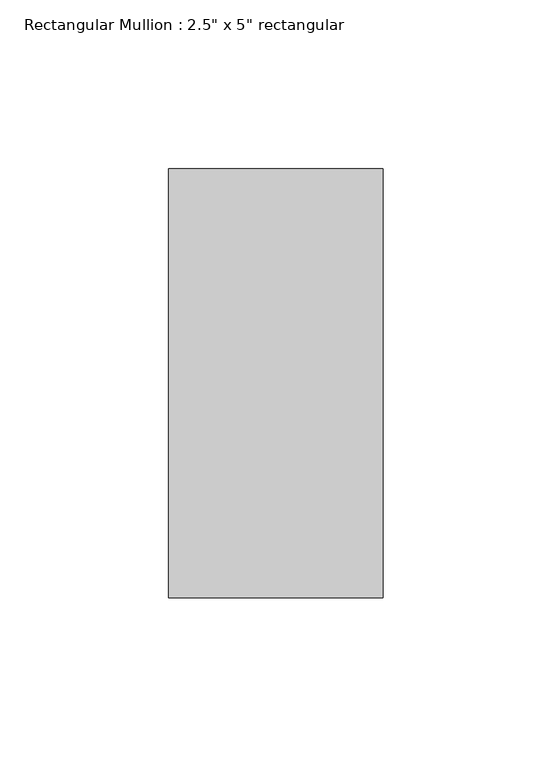
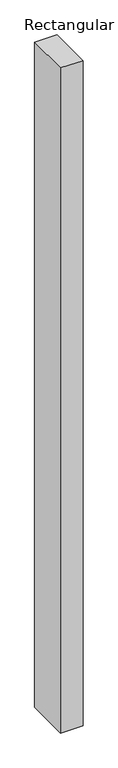
"""IFC4 building model written with IfcOpenShell, lengths in millimetres: member geometry."""

from ifc_helpers import new_model, si_unit, frame, origin, place, context, project, spatial, polyline, outline, extrude, source, transform, mapped, element, save


def member_80b18894(model_context):
    return source(origin(), model_context, "Body", "SweptSolid", [
        extrude(outline(polyline([(0.0, 63.5), (0.0, -63.5), (-63.5, -63.5), (-63.5, 63.5), (0.0, 63.5)])), frame((0.0, 0.0, -1995.867321), z_axis=(0.0, 0.0, 1.0), x_axis=(1.0, 0.0, 0.0)), (0.0, 0.0, 1.0), 1995.867321),
    ])


if __name__ == "__main__":
    model = new_model("IFC4")
    model_context = context("Model", 3, world=origin())
    ifc_project = project(units=[si_unit("LENGTHUNIT", "METRE", prefix="MILLI")], contexts=[model_context])
    site = spatial("IfcSite", under=ifc_project)
    building = spatial("IfcBuilding", under=site)
    placement = place(None, origin())
    member_shape = member_80b18894(model_context)
    element("IfcMember", 1, ObjectType="Rectangular Mullion : 2.5\" x 5\" rectangular", at=placement, inside=building, context=model_context, shape_type="MappedRepresentation", body=[
        mapped(member_shape, transform((0.0, 0.0, 0.0), x_axis=(1.0, 0.0, 0.0), y_axis=(0.0, 1.0, 0.0), z_axis=(0.0, 0.0, 1.0))),
    ])
    save(model, "model.ifc")

# Revit data of these elements
# Type "Rectangular Mullion : 2.5\" x 5\" rectangular"
#   built-in parameter 1007304 = 0.416667 (stored number, unit not read)
#   built-in parameter 1007301 = 0.104167 (stored number, unit not read)
#   built-in parameter 1007300 = 0.104167 (stored number, unit not read)
# Element 1 (IfcMember, "Rectangular Mullion : 2.5\" x 5\" rectangular")
#   Materials on its faces: "Aluminum"
# Materials
#   "Aluminum": class "Metal", colour RGB 247 247 247, transparency 0, Description = "Aluminum 6061", Cost = 0
